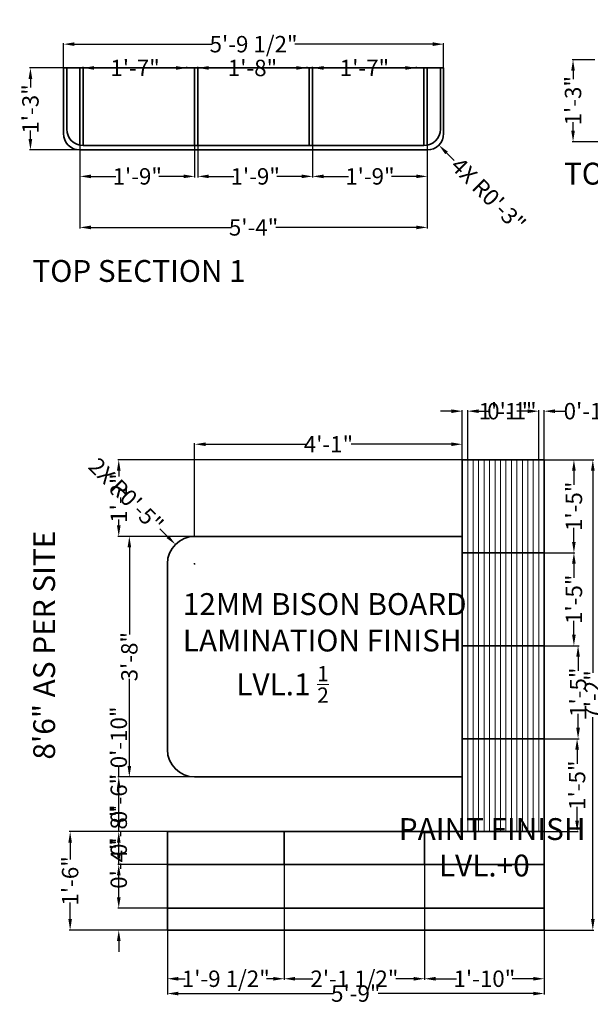
# Model space of a CAD drawing. Units: inches. Extents: x 5 to 197, y 46 to 234.
# Tile 1 of 2: x 5 to 109, y 53 to 233. Entities that reach past the tile are written whole.
import ezdxf

# ---------------------------------------------------------------- set-up
doc = ezdxf.new("R2010")
doc.units = ezdxf.units.IN
doc.header["$MEASUREMENT"] = 0
for name, color, linetype, lineweight in [('A-ANNO-DIMS', 2, 'Continuous', 18), ('A-ANNO-TEXT', 3, 'Continuous', 18), ('A-ELEV', 7, 'Continuous', 35), ('A-ELEV-PATT', 8, 'Continuous', 13), ('A-SECT', 7, 'Continuous', 35)]:
    doc.layers.add(name, color=color, linetype=linetype, lineweight=lineweight)
doc.styles.get("Standard").update_dxf_attribs({"font": 'arial.ttf'})
doc.dimstyles.get("Standard").update_dxf_attribs({"dimtxt": 3, "dimasz": 2, "dimexe": 0.18, "dimexo": 0.0625, "dimgap": 0.09, "dimtad": 0, "dimdec": 0, "dimzin": 0, "dimdsep": 46, "dimlunit": 4, "dimtxsty": 'Standard', "dimcen": 0.09, "dimadec": 0, "dimazin": 0, "dimtfac": 1, "dimtdec": 0, "dimtofl": 0, "dimtmove": 0, "dimatfit": 3, "dimfxl": 1, "dimtolj": 1, "dimtzin": 0, "dimarcsym": 1})

# ---------------------------------------------------------------- blocks, each defined once
blk = doc.blocks.new('*D1')
at = {"layer": 'A-ANNO-DIMS', "color": 0, "lineweight": -2, "transparency": 16777216}
for p, q in [((15.56, 209.27), (15.56, 194.99)), ((79.16, 209.27), (79.16, 194.99)), ((17.56, 195.17), (43.29, 195.17)), ((77.16, 195.17), (51.44, 195.17))]:
    blk.add_line(p, q, dxfattribs=at)
at = {"layer": 'A-ANNO-DIMS', "color": 0, "transparency": 16777216}
for points in [[(17.56, 195.5), (17.56, 194.83), (15.56, 195.17)], [(77.16, 195.5), (77.16, 194.83), (79.16, 195.17)]]:
    blk.add_solid(points, dxfattribs=at)
at = {"layer": 'Defpoints', "color": 0, "transparency": 16777216}
for p in [(15.56, 209.33), (79.16, 209.33), (79.16, 195.17)]:
    blk.add_point(p, dxfattribs=at)
at = {"layer": 'A-ANNO-DIMS', "color": 0, "transparency": 16777216, "insert": (47.36, 195.17), "char_height": 3, "attachment_point": 5}
blk.add_mtext('\\A1;5\'-4"', dxfattribs=at)
blk = doc.blocks.new('*D2')
at = {"layer": 'A-ANNO-DIMS', "color": 0, "lineweight": -2, "transparency": 16777216}
for p, q in [((15.56, 210.07), (15.56, 204.32)), ((36.56, 210.07), (36.56, 204.32)), ((17.56, 204.5), (22.13, 204.5)), ((34.56, 204.5), (30, 204.5))]:
    blk.add_line(p, q, dxfattribs=at)
at = {"layer": 'A-ANNO-DIMS', "color": 0, "transparency": 16777216}
for points in [[(17.56, 204.83), (17.56, 204.17), (15.56, 204.5)], [(34.56, 204.83), (34.56, 204.17), (36.56, 204.5)]]:
    blk.add_solid(points, dxfattribs=at)
at = {"layer": 'Defpoints', "color": 0, "transparency": 16777216}
for p in [(15.56, 210.13), (36.56, 210.13), (36.56, 204.5)]:
    blk.add_point(p, dxfattribs=at)
at = {"layer": 'A-ANNO-DIMS', "color": 0, "transparency": 16777216, "insert": (26.06, 204.5), "char_height": 3, "attachment_point": 5}
blk.add_mtext('\\A1;1\'-9"', dxfattribs=at)
blk = doc.blocks.new('*D3')
at = {"layer": 'A-ANNO-DIMS', "color": 0, "lineweight": -2, "transparency": 16777216}
for p, q in [((37.16, 210.07), (37.16, 204.32)), ((58.16, 210.07), (58.16, 204.32)), ((39.16, 204.5), (43.73, 204.5)), ((56.16, 204.5), (51.6, 204.5))]:
    blk.add_line(p, q, dxfattribs=at)
at = {"layer": 'A-ANNO-DIMS', "color": 0, "transparency": 16777216}
for points in [[(39.16, 204.83), (39.16, 204.17), (37.16, 204.5)], [(56.16, 204.83), (56.16, 204.17), (58.16, 204.5)]]:
    blk.add_solid(points, dxfattribs=at)
at = {"layer": 'Defpoints', "color": 0, "transparency": 16777216}
for p in [(37.16, 210.13), (58.16, 210.13), (58.16, 204.5)]:
    blk.add_point(p, dxfattribs=at)
at = {"layer": 'A-ANNO-DIMS', "color": 0, "transparency": 16777216, "insert": (47.66, 204.5), "char_height": 3, "attachment_point": 5}
blk.add_mtext('\\A1;1\'-9"', dxfattribs=at)
blk = doc.blocks.new('*D4')
at = {"layer": 'A-ANNO-DIMS', "color": 0, "lineweight": -2, "transparency": 16777216}
for p, q in [((58.16, 210.07), (58.16, 204.32)), ((79.16, 210.13), (79.16, 204.32)), ((60.16, 204.5), (64.73, 204.5)), ((77.16, 204.5), (72.6, 204.5))]:
    blk.add_line(p, q, dxfattribs=at)
at = {"layer": 'A-ANNO-DIMS', "color": 0, "transparency": 16777216}
for points in [[(60.16, 204.83), (60.16, 204.17), (58.16, 204.5)], [(77.16, 204.83), (77.16, 204.17), (79.16, 204.5)]]:
    blk.add_solid(points, dxfattribs=at)
at = {"layer": 'Defpoints', "color": 0, "transparency": 16777216}
for p in [(58.16, 210.13), (79.16, 210.19), (79.16, 204.5)]:
    blk.add_point(p, dxfattribs=at)
at = {"layer": 'A-ANNO-DIMS', "color": 0, "transparency": 16777216, "insert": (68.66, 204.5), "char_height": 3, "attachment_point": 5}
blk.add_mtext('\\A1;1\'-9"', dxfattribs=at)
blk = doc.blocks.new('*D5')
at = {"layer": 'A-ANNO-DIMS', "color": 0, "lineweight": -2, "transparency": 16777216}
for p, q in [((16.16, 224.4), (16.16, 224.51)), ((18.16, 224.33), (21.73, 224.33)), ((33.16, 224.33), (29.6, 224.33)), ((35.16, 224.4), (35.16, 224.51))]:
    blk.add_line(p, q, dxfattribs=at)
at = {"layer": 'A-ANNO-DIMS', "color": 0, "transparency": 16777216}
for points in [[(18.16, 224.67), (18.16, 224), (16.16, 224.33)], [(33.16, 224.67), (33.16, 224), (35.16, 224.33)]]:
    blk.add_solid(points, dxfattribs=at)
at = {"layer": 'Defpoints', "color": 0, "transparency": 16777216}
for p in [(16.16, 224.33), (35.16, 224.33), (35.16, 224.33)]:
    blk.add_point(p, dxfattribs=at)
at = {"layer": 'A-ANNO-DIMS', "color": 0, "transparency": 16777216, "insert": (25.66, 224.33), "char_height": 3, "attachment_point": 5}
blk.add_mtext('\\A1;1\'-7"', dxfattribs=at)
blk = doc.blocks.new('*D6')
at = {"layer": 'A-ANNO-DIMS', "color": 0, "lineweight": -2, "transparency": 16777216}
for p, q in [((37.16, 224.4), (37.16, 224.51)), ((39.16, 224.33), (43.23, 224.33)), ((55.16, 224.33), (51.1, 224.33)), ((57.16, 224.4), (57.16, 224.51))]:
    blk.add_line(p, q, dxfattribs=at)
at = {"layer": 'A-ANNO-DIMS', "color": 0, "transparency": 16777216}
for points in [[(39.16, 224.67), (39.16, 224), (37.16, 224.33)], [(55.16, 224.67), (55.16, 224), (57.16, 224.33)]]:
    blk.add_solid(points, dxfattribs=at)
at = {"layer": 'Defpoints', "color": 0, "transparency": 16777216}
for p in [(37.16, 224.33), (57.16, 224.33), (57.16, 224.33)]:
    blk.add_point(p, dxfattribs=at)
at = {"layer": 'A-ANNO-DIMS', "color": 0, "transparency": 16777216, "insert": (47.16, 224.33), "char_height": 3, "attachment_point": 5}
blk.add_mtext('\\A1;1\'-8"', dxfattribs=at)
blk = doc.blocks.new('*D7')
at = {"layer": 'A-ANNO-DIMS', "color": 0, "lineweight": -2, "transparency": 16777216}
for p, q in [((58.16, 224.4), (58.16, 224.51)), ((60.16, 224.33), (63.73, 224.33)), ((75.16, 224.33), (71.6, 224.33)), ((77.16, 224.4), (77.16, 224.51))]:
    blk.add_line(p, q, dxfattribs=at)
at = {"layer": 'A-ANNO-DIMS', "color": 0, "transparency": 16777216}
for points in [[(60.16, 224.67), (60.16, 224), (58.16, 224.33)], [(75.16, 224.67), (75.16, 224), (77.16, 224.33)]]:
    blk.add_solid(points, dxfattribs=at)
at = {"layer": 'Defpoints', "color": 0, "transparency": 16777216}
for p in [(58.16, 224.33), (77.16, 224.33), (77.16, 224.33)]:
    blk.add_point(p, dxfattribs=at)
at = {"layer": 'A-ANNO-DIMS', "color": 0, "transparency": 16777216, "insert": (67.66, 224.33), "char_height": 3, "attachment_point": 5}
blk.add_mtext('\\A1;1\'-7"', dxfattribs=at)
blk = doc.blocks.new('*D8')
at = {"layer": 'A-ANNO-DIMS', "color": 0, "lineweight": -2, "transparency": 16777216}
for p, q in [((16.1, 224.33), (6.32, 224.33)), ((6.5, 222.33), (6.5, 220.77)), ((6.5, 211.33), (6.5, 212.9)), ((15.5, 209.33), (6.32, 209.33))]:
    blk.add_line(p, q, dxfattribs=at)
at = {"layer": 'A-ANNO-DIMS', "color": 0, "transparency": 16777216}
for points in [[(6.16, 222.33), (6.83, 222.33), (6.5, 224.33)], [(6.16, 211.33), (6.83, 211.33), (6.5, 209.33)]]:
    blk.add_solid(points, dxfattribs=at)
at = {"layer": 'Defpoints', "color": 0, "transparency": 16777216}
for p in [(16.16, 224.33), (6.5, 209.33), (15.56, 209.33)]:
    blk.add_point(p, dxfattribs=at)
at = {"layer": 'A-ANNO-DIMS', "color": 0, "transparency": 16777216, "insert": (6.5, 216.83), "char_height": 3, "attachment_point": 5, "rotation": 90}
blk.add_mtext('\\A1;1\'-3"', dxfattribs=at)
blk = doc.blocks.new('*D9')
at = {"layer": 'A-ANNO-DIMS', "color": 0, "lineweight": -2, "transparency": 16777216}
for p, q in [((100.64, 135.66), (106.19, 135.66)), ((106.01, 133.66), (106.01, 131.09)), ((106.01, 120.66), (106.01, 123.22)), ((100.64, 118.66), (106.19, 118.66))]:
    blk.add_line(p, q, dxfattribs=at)
at = {"layer": 'A-ANNO-DIMS', "color": 0, "transparency": 16777216}
for points in [[(105.67, 133.66), (106.34, 133.66), (106.01, 135.66)], [(105.67, 120.66), (106.34, 120.66), (106.01, 118.66)]]:
    blk.add_solid(points, dxfattribs=at)
at = {"layer": 'Defpoints', "color": 0, "transparency": 16777216}
for p in [(100.57, 135.66), (106.01, 135.66), (100.57, 118.66)]:
    blk.add_point(p, dxfattribs=at)
at = {"layer": 'A-ANNO-DIMS', "color": 0, "transparency": 16777216, "insert": (106.01, 127.16), "char_height": 3, "attachment_point": 5, "rotation": 90}
blk.add_mtext('\\A1;1\'-5"', dxfattribs=at)
blk = doc.blocks.new('*D10')
at = {"layer": 'A-ANNO-DIMS', "color": 0, "lineweight": -2, "transparency": 16777216}
for p, q in [((100.64, 118.66), (106.95, 118.66)), ((106.77, 116.66), (106.77, 114.09)), ((106.77, 103.66), (106.77, 106.22)), ((100.64, 101.66), (106.95, 101.66))]:
    blk.add_line(p, q, dxfattribs=at)
at = {"layer": 'A-ANNO-DIMS', "color": 0, "transparency": 16777216}
for points in [[(106.44, 116.66), (107.11, 116.66), (106.77, 118.66)], [(106.44, 103.66), (107.11, 103.66), (106.77, 101.66)]]:
    blk.add_solid(points, dxfattribs=at)
at = {"layer": 'Defpoints', "color": 0, "transparency": 16777216}
for p in [(100.57, 118.66), (106.77, 118.66), (100.57, 101.66)]:
    blk.add_point(p, dxfattribs=at)
at = {"layer": 'A-ANNO-DIMS', "color": 0, "transparency": 16777216, "insert": (106.77, 110.16), "char_height": 3, "attachment_point": 5, "rotation": 90}
blk.add_mtext('\\A1;1\'-5"', dxfattribs=at)
blk = doc.blocks.new('*D11')
at = {"layer": 'A-ANNO-DIMS', "color": 0, "lineweight": -2, "transparency": 16777216}
for p, q in [((100.64, 101.66), (106.77, 101.66)), ((106.59, 99.66), (106.59, 97.09)), ((106.59, 86.66), (106.59, 89.22)), ((100.64, 84.66), (106.77, 84.66))]:
    blk.add_line(p, q, dxfattribs=at)
at = {"layer": 'A-ANNO-DIMS', "color": 0, "transparency": 16777216}
for points in [[(106.26, 99.66), (106.93, 99.66), (106.59, 101.66)], [(106.26, 86.66), (106.93, 86.66), (106.59, 84.66)]]:
    blk.add_solid(points, dxfattribs=at)
at = {"layer": 'Defpoints', "color": 0, "transparency": 16777216}
for p in [(100.57, 101.66), (106.59, 101.66), (100.57, 84.66)]:
    blk.add_point(p, dxfattribs=at)
at = {"layer": 'A-ANNO-DIMS', "color": 0, "transparency": 16777216, "insert": (106.59, 93.16), "char_height": 3, "attachment_point": 5, "rotation": 90}
blk.add_mtext('\\A1;1\'-5"', dxfattribs=at)
blk = doc.blocks.new('*D12')
at = {"layer": 'A-ANNO-DIMS', "color": 0, "lineweight": -2, "transparency": 16777216}
for p, q in [((31.57, 66.59), (31.57, 54.87)), ((100.57, 66.59), (100.57, 54.87)), ((33.57, 55.05), (62, 55.05)), ((98.57, 55.05), (70.15, 55.05))]:
    blk.add_line(p, q, dxfattribs=at)
at = {"layer": 'A-ANNO-DIMS', "color": 0, "transparency": 16777216}
for points in [[(33.57, 55.38), (33.57, 54.72), (31.57, 55.05)], [(98.57, 55.38), (98.57, 54.72), (100.57, 55.05)]]:
    blk.add_solid(points, dxfattribs=at)
at = {"layer": 'Defpoints', "color": 0, "transparency": 16777216}
for p in [(31.57, 66.66), (100.57, 66.66), (31.57, 55.05)]:
    blk.add_point(p, dxfattribs=at)
at = {"layer": 'A-ANNO-DIMS', "color": 0, "transparency": 16777216, "insert": (66.07, 55.05), "char_height": 3, "attachment_point": 5}
blk.add_mtext('\\A1;5\'-9"', dxfattribs=at)
blk = doc.blocks.new('*D13')
at = {"layer": 'A-ANNO-DIMS', "color": 0, "lineweight": -2, "transparency": 16777216}
for p, q in [((31.51, 84.66), (13.59, 84.66)), ((13.77, 82.66), (13.77, 79.59)), ((13.77, 68.66), (13.77, 71.72)), ((31.51, 66.66), (13.59, 66.66))]:
    blk.add_line(p, q, dxfattribs=at)
at = {"layer": 'A-ANNO-DIMS', "color": 0, "transparency": 16777216}
for points in [[(13.44, 82.66), (14.1, 82.66), (13.77, 84.66)], [(13.44, 68.66), (14.1, 68.66), (13.77, 66.66)]]:
    blk.add_solid(points, dxfattribs=at)
at = {"layer": 'Defpoints', "color": 0, "transparency": 16777216}
for p in [(13.77, 84.66), (31.57, 84.66), (31.57, 66.66)]:
    blk.add_point(p, dxfattribs=at)
at = {"layer": 'A-ANNO-DIMS', "color": 0, "transparency": 16777216, "insert": (13.77, 75.66), "char_height": 3, "attachment_point": 5, "rotation": 90}
blk.add_mtext('\\A1;1\'-6"', dxfattribs=at)
blk = doc.blocks.new('*D14')
at = {"layer": 'A-ANNO-DIMS', "color": 0, "lineweight": -2, "transparency": 16777216}
for p, q in [((100.64, 152.66), (106.19, 152.66)), ((106.01, 150.66), (106.01, 148.09)), ((106.01, 137.66), (106.01, 140.22)), ((100.64, 135.66), (106.19, 135.66))]:
    blk.add_line(p, q, dxfattribs=at)
at = {"layer": 'A-ANNO-DIMS', "color": 0, "transparency": 16777216}
for points in [[(105.67, 150.66), (106.34, 150.66), (106.01, 152.66)], [(105.67, 137.66), (106.34, 137.66), (106.01, 135.66)]]:
    blk.add_solid(points, dxfattribs=at)
at = {"layer": 'Defpoints', "color": 0, "transparency": 16777216}
for p in [(100.57, 152.66), (106.01, 152.66), (100.57, 135.66)]:
    blk.add_point(p, dxfattribs=at)
at = {"layer": 'A-ANNO-DIMS', "color": 0, "transparency": 16777216, "insert": (106.01, 144.16), "char_height": 3, "attachment_point": 5, "rotation": 90}
blk.add_mtext('\\A1;1\'-5"', dxfattribs=at)
blk = doc.blocks.new('*D15')
at = {"layer": 'A-ANNO-DIMS', "color": 0, "lineweight": -2, "transparency": 16777216}
for p, q in [((36.51, 138.66), (24.43, 138.66)), ((24.61, 136.66), (24.61, 120.73)), ((24.61, 96.66), (24.61, 112.58)), ((36.51, 94.66), (24.43, 94.66))]:
    blk.add_line(p, q, dxfattribs=at)
at = {"layer": 'A-ANNO-DIMS', "color": 0, "transparency": 16777216}
for points in [[(24.28, 136.66), (24.94, 136.66), (24.61, 138.66)], [(24.28, 96.66), (24.94, 96.66), (24.61, 94.66)]]:
    blk.add_solid(points, dxfattribs=at)
at = {"layer": 'Defpoints', "color": 0, "transparency": 16777216}
for p in [(36.57, 138.66), (24.61, 94.66), (36.57, 94.66)]:
    blk.add_point(p, dxfattribs=at)
at = {"layer": 'A-ANNO-DIMS', "color": 0, "transparency": 16777216, "insert": (24.61, 116.66), "char_height": 3, "attachment_point": 5, "rotation": 90}
blk.add_mtext('\\A1;3\'-8"', dxfattribs=at)
blk = doc.blocks.new('*D16')
at = {"layer": 'A-ANNO-DIMS', "color": 0, "lineweight": -2, "transparency": 16777216}
for p, q in [((36.57, 138.72), (36.57, 155.69)), ((38.57, 155.51), (56.94, 155.51)), ((83.57, 155.51), (65.21, 155.51)), ((85.57, 138.72), (85.57, 155.69))]:
    blk.add_line(p, q, dxfattribs=at)
at = {"layer": 'A-ANNO-DIMS', "color": 0, "transparency": 16777216}
for points in [[(38.57, 155.84), (38.57, 155.18), (36.57, 155.51)], [(83.57, 155.84), (83.57, 155.18), (85.57, 155.51)]]:
    blk.add_solid(points, dxfattribs=at)
at = {"layer": 'Defpoints', "color": 0, "transparency": 16777216}
for p in [(85.57, 155.51), (36.57, 138.66), (85.57, 138.66)]:
    blk.add_point(p, dxfattribs=at)
at = {"layer": 'A-ANNO-DIMS', "color": 0, "transparency": 16777216, "insert": (61.07, 155.51), "char_height": 3, "attachment_point": 5}
blk.add_mtext('\\A1;4\'-1"', dxfattribs=at)
blk = doc.blocks.new('*D17')
at = {"layer": 'A-ANNO-DIMS', "color": 0, "lineweight": -2, "transparency": 16777216}
for p, q in [((22.67, 72.66), (22.67, 74.66)), ((31.51, 70.66), (22.49, 70.66)), ((31.51, 66.66), (22.49, 66.66)), ((22.67, 64.66), (22.67, 62.66))]:
    blk.add_line(p, q, dxfattribs=at)
at = {"layer": 'A-ANNO-DIMS', "color": 0, "transparency": 16777216}
for points in [[(22.34, 72.66), (23.01, 72.66), (22.67, 70.66)], [(22.34, 64.66), (23.01, 64.66), (22.67, 66.66)]]:
    blk.add_solid(points, dxfattribs=at)
at = {"layer": 'Defpoints', "color": 0, "transparency": 16777216}
for p in [(22.67, 70.66), (31.57, 70.66), (31.57, 66.66)]:
    blk.add_point(p, dxfattribs=at)
at = {"layer": 'A-ANNO-DIMS', "color": 0, "transparency": 16777216, "insert": (22.67, 78.73), "char_height": 3, "attachment_point": 5, "rotation": 90}
blk.add_mtext('\\A1;0\'-4"', dxfattribs=at)
blk = doc.blocks.new('*D18')
at = {"layer": 'A-ANNO-DIMS', "color": 0, "lineweight": -2, "transparency": 16777216}
for p, q in [((22.67, 78.66), (22.67, 80.66)), ((31.51, 78.66), (22.49, 78.66)), ((22.67, 72.66), (22.67, 76.66)), ((31.51, 70.66), (22.49, 70.66))]:
    blk.add_line(p, q, dxfattribs=at)
at = {"layer": 'A-ANNO-DIMS', "color": 0, "transparency": 16777216}
for points in [[(22.34, 76.66), (23.01, 76.66), (22.67, 78.66)], [(22.34, 72.66), (23.01, 72.66), (22.67, 70.66)]]:
    blk.add_solid(points, dxfattribs=at)
at = {"layer": 'Defpoints', "color": 0, "transparency": 16777216}
for p in [(22.67, 78.66), (31.57, 78.66), (31.57, 70.66)]:
    blk.add_point(p, dxfattribs=at)
at = {"layer": 'A-ANNO-DIMS', "color": 0, "transparency": 16777216, "insert": (22.67, 84.73), "char_height": 3, "attachment_point": 5, "rotation": 90}
blk.add_mtext('\\A1;0\'-8"', dxfattribs=at)
blk = doc.blocks.new('*D19')
at = {"layer": 'A-ANNO-DIMS', "color": 0, "lineweight": -2, "transparency": 16777216}
for p, q in [((22.67, 84.66), (22.67, 86.66)), ((31.51, 84.66), (22.49, 84.66)), ((22.67, 80.66), (22.67, 82.66)), ((31.51, 78.66), (22.49, 78.66))]:
    blk.add_line(p, q, dxfattribs=at)
at = {"layer": 'A-ANNO-DIMS', "color": 0, "transparency": 16777216}
for points in [[(22.34, 82.66), (23.01, 82.66), (22.67, 84.66)], [(22.34, 80.66), (23.01, 80.66), (22.67, 78.66)]]:
    blk.add_solid(points, dxfattribs=at)
at = {"layer": 'Defpoints', "color": 0, "transparency": 16777216}
for p in [(22.67, 84.66), (31.57, 84.66), (31.57, 78.66)]:
    blk.add_point(p, dxfattribs=at)
at = {"layer": 'A-ANNO-DIMS', "color": 0, "transparency": 16777216, "insert": (22.67, 90.73), "char_height": 3, "attachment_point": 5, "rotation": 90}
blk.add_mtext('\\A1;0\'-6"', dxfattribs=at)
blk = doc.blocks.new('*D20')
at = {"layer": 'A-ANNO-DIMS', "color": 0, "lineweight": -2, "transparency": 16777216}
for p, q in [((22.67, 94.66), (22.67, 96.66)), ((36.51, 94.66), (22.49, 94.66)), ((22.67, 86.66), (22.67, 92.66)), ((31.51, 84.66), (22.49, 84.66))]:
    blk.add_line(p, q, dxfattribs=at)
at = {"layer": 'A-ANNO-DIMS', "color": 0, "transparency": 16777216}
for points in [[(22.34, 92.66), (23.01, 92.66), (22.67, 94.66)], [(22.34, 86.66), (23.01, 86.66), (22.67, 84.66)]]:
    blk.add_solid(points, dxfattribs=at)
at = {"layer": 'Defpoints', "color": 0, "transparency": 16777216}
for p in [(22.67, 94.66), (36.57, 94.66), (31.57, 84.66)]:
    blk.add_point(p, dxfattribs=at)
at = {"layer": 'A-ANNO-DIMS', "color": 0, "transparency": 16777216, "insert": (22.67, 101.9), "char_height": 3, "attachment_point": 5, "rotation": 90}
blk.add_mtext('\\A1;0\'-10"', dxfattribs=at)
blk = doc.blocks.new('*D21')
at = {"layer": 'A-ANNO-DIMS', "color": 0, "lineweight": -2, "transparency": 16777216}
for p, q in [((85.51, 152.66), (22.49, 152.66)), ((22.67, 150.66), (22.67, 149.59)), ((22.67, 140.66), (22.67, 141.72)), ((36.51, 138.66), (22.49, 138.66))]:
    blk.add_line(p, q, dxfattribs=at)
at = {"layer": 'A-ANNO-DIMS', "color": 0, "transparency": 16777216}
for points in [[(22.34, 150.66), (23.01, 150.66), (22.67, 152.66)], [(22.34, 140.66), (23.01, 140.66), (22.67, 138.66)]]:
    blk.add_solid(points, dxfattribs=at)
at = {"layer": 'Defpoints', "color": 0, "transparency": 16777216}
for p in [(22.67, 152.66), (85.57, 152.66), (36.57, 138.66)]:
    blk.add_point(p, dxfattribs=at)
at = {"layer": 'A-ANNO-DIMS', "color": 0, "transparency": 16777216, "insert": (22.67, 145.66), "char_height": 3, "attachment_point": 5, "rotation": 90}
blk.add_mtext('\\A1;1\'-2"', dxfattribs=at)
blk = doc.blocks.new('*D22')
at = {"layer": 'A-ANNO-DIMS', "color": 0, "lineweight": -2, "transparency": 16777216}
for p, q in [((100.64, 152.66), (109.65, 152.66)), ((109.47, 150.66), (109.47, 113.72)), ((109.47, 68.66), (109.47, 105.59)), ((100.64, 66.66), (109.65, 66.66))]:
    blk.add_line(p, q, dxfattribs=at)
at = {"layer": 'A-ANNO-DIMS', "color": 0, "transparency": 16777216}
for points in [[(109.14, 150.66), (109.81, 150.66), (109.47, 152.66)], [(109.14, 68.66), (109.81, 68.66), (109.47, 66.66)]]:
    blk.add_solid(points, dxfattribs=at)
at = {"layer": 'Defpoints', "color": 0, "transparency": 16777216}
for p in [(100.57, 152.66), (109.47, 152.66), (100.57, 66.66)]:
    blk.add_point(p, dxfattribs=at)
at = {"layer": 'A-ANNO-DIMS', "color": 0, "transparency": 16777216, "insert": (109.47, 109.66), "char_height": 3, "attachment_point": 5, "rotation": 90}
blk.add_mtext('\\A1;7\'-2"', dxfattribs=at)
blk = doc.blocks.new('*D23')
at = {"layer": 'A-ANNO-DIMS', "color": 0, "lineweight": -2, "transparency": 16777216}
for p, q in [((31.57, 84.59), (31.57, 57.58)), ((52.97, 84.59), (52.97, 57.58)), ((33.57, 57.76), (34.84, 57.76)), ((50.97, 57.76), (49.7, 57.76))]:
    blk.add_line(p, q, dxfattribs=at)
at = {"layer": 'A-ANNO-DIMS', "color": 0, "transparency": 16777216}
for points in [[(33.57, 58.09), (33.57, 57.42), (31.57, 57.76)], [(50.97, 58.09), (50.97, 57.42), (52.97, 57.76)]]:
    blk.add_solid(points, dxfattribs=at)
at = {"layer": 'Defpoints', "color": 0, "transparency": 16777216}
for p in [(31.57, 84.66), (52.97, 84.66), (52.97, 57.76)]:
    blk.add_point(p, dxfattribs=at)
at = {"layer": 'A-ANNO-DIMS', "color": 0, "transparency": 16777216, "insert": (42.27, 57.76), "char_height": 3, "attachment_point": 5}
blk.add_mtext('\\A1;1\'-9 1/2"', dxfattribs=at)
blk = doc.blocks.new('*D24')
at = {"layer": 'A-ANNO-DIMS', "color": 0, "lineweight": -2, "transparency": 16777216}
for p, q in [((52.97, 84.59), (52.97, 57.58)), ((78.67, 84.59), (78.67, 57.58)), ((54.97, 57.76), (58.22, 57.76)), ((76.67, 57.76), (73.41, 57.76))]:
    blk.add_line(p, q, dxfattribs=at)
at = {"layer": 'A-ANNO-DIMS', "color": 0, "transparency": 16777216}
for points in [[(54.97, 58.09), (54.97, 57.42), (52.97, 57.76)], [(76.67, 58.09), (76.67, 57.42), (78.67, 57.76)]]:
    blk.add_solid(points, dxfattribs=at)
at = {"layer": 'Defpoints', "color": 0, "transparency": 16777216}
for p in [(52.97, 84.66), (78.67, 84.66), (78.67, 57.76)]:
    blk.add_point(p, dxfattribs=at)
at = {"layer": 'A-ANNO-DIMS', "color": 0, "transparency": 16777216, "insert": (65.82, 57.76), "char_height": 3, "attachment_point": 5}
blk.add_mtext('\\A1;2\'-1 1/2"', dxfattribs=at)
blk = doc.blocks.new('*D25')
at = {"layer": 'A-ANNO-DIMS', "color": 0, "lineweight": -2, "transparency": 16777216}
for p, q in [((78.67, 84.59), (78.67, 57.58)), ((100.57, 84.59), (100.57, 57.58)), ((80.67, 57.76), (84.52, 57.76)), ((98.57, 57.76), (94.72, 57.76))]:
    blk.add_line(p, q, dxfattribs=at)
at = {"layer": 'A-ANNO-DIMS', "color": 0, "transparency": 16777216}
for points in [[(80.67, 58.09), (80.67, 57.42), (78.67, 57.76)], [(98.57, 58.09), (98.57, 57.42), (100.57, 57.76)]]:
    blk.add_solid(points, dxfattribs=at)
at = {"layer": 'Defpoints', "color": 0, "transparency": 16777216}
for p in [(78.67, 84.66), (100.57, 84.66), (100.57, 57.76)]:
    blk.add_point(p, dxfattribs=at)
at = {"layer": 'A-ANNO-DIMS', "color": 0, "transparency": 16777216, "insert": (89.62, 57.76), "char_height": 3, "attachment_point": 5}
blk.add_mtext('\\A1;1\'-10"', dxfattribs=at)
blk = doc.blocks.new('*D26')
at = {"layer": 'A-ANNO-DIMS', "color": 0, "lineweight": -2, "transparency": 16777216}
for p, q in [((83.57, 161.56), (81.57, 161.56)), ((85.57, 152.72), (85.57, 161.74)), ((86.57, 152.72), (86.57, 161.74)), ((88.57, 161.56), (90.57, 161.56))]:
    blk.add_line(p, q, dxfattribs=at)
at = {"layer": 'A-ANNO-DIMS', "color": 0, "transparency": 16777216}
for points in [[(83.57, 161.89), (83.57, 161.22), (85.57, 161.56)], [(88.57, 161.89), (88.57, 161.22), (86.57, 161.56)]]:
    blk.add_solid(points, dxfattribs=at)
at = {"layer": 'Defpoints', "color": 0, "transparency": 16777216}
for p in [(86.57, 161.56), (85.57, 152.66), (86.57, 152.66)]:
    blk.add_point(p, dxfattribs=at)
at = {"layer": 'A-ANNO-DIMS', "color": 0, "transparency": 16777216, "insert": (94.65, 161.56), "char_height": 3, "attachment_point": 5}
blk.add_mtext('\\A1;0\'-1"', dxfattribs=at)
blk = doc.blocks.new('*D27')
at = {"layer": 'A-ANNO-DIMS', "color": 0, "lineweight": -2, "transparency": 16777216}
for p, q in [((86.57, 152.72), (86.57, 161.74)), ((88.57, 161.56), (89.14, 161.56)), ((97.57, 161.56), (97.01, 161.56)), ((99.57, 152.72), (99.57, 161.74))]:
    blk.add_line(p, q, dxfattribs=at)
at = {"layer": 'A-ANNO-DIMS', "color": 0, "transparency": 16777216}
for points in [[(88.57, 161.89), (88.57, 161.22), (86.57, 161.56)], [(97.57, 161.89), (97.57, 161.22), (99.57, 161.56)]]:
    blk.add_solid(points, dxfattribs=at)
at = {"layer": 'Defpoints', "color": 0, "transparency": 16777216}
for p in [(99.57, 161.56), (86.57, 152.66), (99.57, 152.66)]:
    blk.add_point(p, dxfattribs=at)
at = {"layer": 'A-ANNO-DIMS', "color": 0, "transparency": 16777216, "insert": (93.07, 161.56), "char_height": 3, "attachment_point": 5}
blk.add_mtext('\\A1;1\'-1"', dxfattribs=at)
blk = doc.blocks.new('*D28')
at = {"layer": 'A-ANNO-DIMS', "color": 0, "lineweight": -2, "transparency": 16777216}
for p, q in [((97.57, 161.56), (95.57, 161.56)), ((99.57, 152.72), (99.57, 161.74)), ((100.57, 152.72), (100.57, 161.74)), ((102.57, 161.56), (104.57, 161.56))]:
    blk.add_line(p, q, dxfattribs=at)
at = {"layer": 'A-ANNO-DIMS', "color": 0, "transparency": 16777216}
for points in [[(97.57, 161.89), (97.57, 161.22), (99.57, 161.56)], [(102.57, 161.89), (102.57, 161.22), (100.57, 161.56)]]:
    blk.add_solid(points, dxfattribs=at)
at = {"layer": 'Defpoints', "color": 0, "transparency": 16777216}
for p in [(100.57, 161.56), (99.57, 152.66), (100.57, 152.66)]:
    blk.add_point(p, dxfattribs=at)
at = {"layer": 'A-ANNO-DIMS', "color": 0, "transparency": 16777216, "insert": (108.65, 161.56), "char_height": 3, "attachment_point": 5}
blk.add_mtext('\\A1;0\'-1"', dxfattribs=at)
blk = doc.blocks.new('*D29')
at = {"layer": 'A-ANNO-DIMS', "color": 0, "lineweight": -2, "transparency": 16777216}
for p, q in [((12.56, 224.4), (12.56, 228.86)), ((82.16, 224.4), (82.16, 228.86)), ((14.56, 228.68), (39.79, 228.68)), ((80.16, 228.68), (54.94, 228.68))]:
    blk.add_line(p, q, dxfattribs=at)
at = {"layer": 'A-ANNO-DIMS', "color": 0, "transparency": 16777216}
for points in [[(14.56, 229.02), (14.56, 228.35), (12.56, 228.68)], [(80.16, 229.02), (80.16, 228.35), (82.16, 228.68)]]:
    blk.add_solid(points, dxfattribs=at)
at = {"layer": 'Defpoints', "color": 0, "transparency": 16777216}
for p in [(82.16, 228.68), (12.56, 224.33), (82.16, 224.33)]:
    blk.add_point(p, dxfattribs=at)
at = {"layer": 'A-ANNO-DIMS', "color": 0, "transparency": 16777216, "insert": (47.36, 228.68), "char_height": 3, "attachment_point": 5}
blk.add_mtext('\\A1;5\'-9 1/2"', dxfattribs=at)
blk = doc.blocks.new('*D33')
at = {"layer": 'A-ANNO-DIMS', "color": 0, "lineweight": -2, "transparency": 16777216}
for p, q in [((109.84, 225.84), (105.67, 225.84)), ((105.85, 223.84), (105.85, 222.27)), ((105.85, 212.84), (105.85, 214.4)), ((112.84, 210.84), (105.67, 210.84))]:
    blk.add_line(p, q, dxfattribs=at)
at = {"layer": 'A-ANNO-DIMS', "color": 0, "transparency": 16777216}
for points in [[(105.52, 223.84), (106.18, 223.84), (105.85, 225.84)], [(105.52, 212.84), (106.18, 212.84), (105.85, 210.84)]]:
    blk.add_solid(points, dxfattribs=at)
at = {"layer": 'Defpoints', "color": 0, "transparency": 16777216}
for p in [(109.9, 225.84), (105.85, 210.84), (112.9, 210.84)]:
    blk.add_point(p, dxfattribs=at)
at = {"layer": 'A-ANNO-DIMS', "color": 0, "transparency": 16777216, "insert": (105.85, 218.34), "char_height": 3, "attachment_point": 5, "rotation": 90}
blk.add_mtext('\\A1;1\'-3"', dxfattribs=at)
blk = doc.blocks.new('*D35')
at = {"layer": 'A-ANNO-DIMS', "color": 0, "lineweight": -2, "transparency": 16777216}
for p, q in [((30.21, 140.02), (31.62, 138.61)), ((36.48, 133.66), (36.66, 133.66)), ((36.57, 133.57), (36.57, 133.75))]:
    blk.add_line(p, q, dxfattribs=at)
at = {"layer": 'A-ANNO-DIMS', "color": 0, "transparency": 16777216}
blk.add_solid([(31.86, 138.84), (31.39, 138.37), (33.04, 137.19)], dxfattribs=at)
at = {"layer": 'Defpoints', "color": 0, "transparency": 16777216}
for p in [(33.04, 137.19), (36.57, 133.66)]:
    blk.add_point(p, dxfattribs=at)
at = {"layer": 'A-ANNO-DIMS', "color": 0, "transparency": 16777216, "insert": (24.01, 146.21), "char_height": 3, "attachment_point": 5, "rotation": 315.007}
blk.add_mtext('\\A1;2X R0\'-5"', dxfattribs=at)
blk = doc.blocks.new('*D36')
at = {"layer": 'A-ANNO-DIMS', "color": 0, "lineweight": -2, "transparency": 16777216}
for p, q in [((79.07, 212.33), (79.25, 212.33)), ((79.16, 212.24), (79.16, 212.42)), ((84.11, 207.38), (82.7, 208.8))]:
    blk.add_line(p, q, dxfattribs=at)
at = {"layer": 'A-ANNO-DIMS', "color": 0, "transparency": 16777216}
blk.add_solid([(82.94, 209.03), (82.46, 208.56), (81.29, 210.21)], dxfattribs=at)
at = {"layer": 'Defpoints', "color": 0, "transparency": 16777216}
for p in [(79.16, 212.33), (81.29, 210.21)]:
    blk.add_point(p, dxfattribs=at)
at = {"layer": 'A-ANNO-DIMS', "color": 0, "transparency": 16777216, "insert": (90.34, 201.16), "char_height": 3, "attachment_point": 5, "rotation": 315.0044}
blk.add_mtext('\\A1;4X R0\'-3"', dxfattribs=at)

msp = doc.modelspace()

# ---------------------------------------------------------------- linework, layer by layer
at = {"layer": 'A-ELEV'}
for p, q in [((85.57, 152.66), (85.57, 84.66)), ((100.57, 152.66), (85.57, 152.66)), ((100.57, 135.66), (100.57, 152.66)), ((36.57, 138.66), (85.57, 138.66)), ((100.57, 135.66), (85.57, 135.66)), ((100.57, 118.66), (100.57, 135.66)), ((31.57, 133.66), (31.57, 99.66)), ((100.57, 118.66), (85.57, 118.66)), ((100.57, 101.66), (100.57, 118.66)), ((100.57, 101.66), (85.57, 101.66)), ((100.57, 84.66), (100.57, 101.66)), ((36.57, 94.66), (85.57, 94.66)), ((31.57, 66.66), (31.57, 84.66)), ((31.57, 84.66), (85.57, 84.66)), ((52.97, 84.66), (52.97, 78.66)), ((78.67, 78.66), (78.67, 84.66)), ((85.57, 84.66), (100.57, 84.66)), ((100.57, 84.66), (100.57, 66.66)), ((100.57, 78.66), (31.57, 78.66)), ((100.57, 70.66), (31.57, 70.66)), ((100.57, 66.66), (31.57, 66.66))]:
    msp.add_line(p, q, dxfattribs=at)
for centre, start, end in [((36.57, 133.66), 90, 180), ((36.57, 99.66), 180, 270)]:
    msp.add_arc(centre, 5, start, end, dxfattribs=at)
at = {"layer": 'A-ELEV-PATT'}
for p, q in [((86.57, 152.66), (86.57, 84.66)), ((87.57, 152.66), (87.57, 84.66)), ((88.57, 152.66), (88.57, 84.66)), ((89.57, 152.66), (89.57, 84.66)), ((90.57, 152.66), (90.57, 84.66)), ((91.57, 152.66), (91.57, 84.66)), ((92.57, 152.66), (92.57, 84.66)), ((93.57, 152.66), (93.57, 84.66)), ((94.57, 152.66), (94.57, 84.66)), ((95.57, 152.66), (95.57, 84.66)), ((96.57, 152.66), (96.57, 84.66)), ((97.57, 152.66), (97.57, 84.66)), ((98.57, 152.66), (98.57, 84.66)), ((99.57, 152.66), (99.57, 84.66))]:
    msp.add_line(p, q, dxfattribs=at)
at = {"layer": 'A-SECT'}
for p, q in [((82.16, 224.33), (12.56, 224.33)), ((12.56, 224.33), (12.56, 212.33)), ((13.16, 224.33), (13.16, 213.13)), ((15.56, 224.33), (15.56, 210.13)), ((16.16, 224.33), (16.16, 210.13)), ((36.56, 224.33), (36.56, 210.13)), ((37.16, 224.33), (37.16, 210.13)), ((57.56, 224.33), (57.56, 210.13)), ((58.16, 224.33), (58.16, 210.13)), ((78.56, 224.33), (78.56, 210.13)), ((79.16, 224.33), (79.16, 210.13)), ((81.56, 224.33), (81.56, 213.13)), ((82.16, 224.33), (82.16, 212.33)), ((15.56, 209.33), (79.16, 209.33)), ((16.16, 210.13), (78.56, 210.13))]:
    msp.add_line(p, q, dxfattribs=at)
for centre, start, end in [((16.16, 213.13), 180, 270), ((78.56, 213.13), 270, 0), ((15.56, 212.33), 180, 270), ((79.16, 212.33), 270, 0)]:
    msp.add_arc(centre, 3, start, end, dxfattribs=at)

# ---------------------------------------------------------------- texts
at = {"layer": 'A-ANNO-TEXT', "char_height": 4, "attachment_point": 1}
for s, width, insert in [('TOP SECTION 2', 72.0117, (104.18, 207)), ('TOP SECTION 1', 52.888, (6.86, 189.2)), ('\\A1;12MM BISON BOARD\\PLAMINATION FINISH\\P        LVL.1 {\\H0.7x;\\S1/2;}', 125.0016, (34.4, 128.28)), ('PAINT FINISH \\P      LVL.+0', 80.2681, (73.95, 87.13))]:
    msp.add_mtext_dynamic_manual_height_columns(s, width=width, gutter_width=20, heights=[0], dxfattribs=dict(at, insert=insert))
at = {"layer": 'A-ANNO-TEXT', "insert": (7.01, 97.84), "char_height": 4, "attachment_point": 1, "rotation": 90}
msp.add_mtext_dynamic_manual_height_columns('8\'6" AS PER SITE', width=115.2159, gutter_width=20, heights=[0], dxfattribs=at)

# ---------------------------------------------------------------- dimensions: what is measured, and where the dimension line sits
at = {"layer": 'A-ANNO-DIMS'}
for base, p1, p2, override, picture, middle in [((82.16, 228.68), (12.56, 224.33), (82.16, 224.33), {"dimdec": 1, "dimlfac": 1, "dimrnd": 0, "dimzin": 1, "dimdsep": 46, "dimlunit": 4, "dimfrac": 2}, '*D29', (47.36, 228.68)), ((35.16, 224.33), (16.16, 224.33), (35.16, 224.33), {"dimclrd": 0, "dimclre": 0, "dimclrt": 0}, '*D5', (25.66, 224.33)), ((57.16, 224.33), (37.16, 224.33), (57.16, 224.33), {"dimclrd": 0, "dimclre": 0, "dimclrt": 0}, '*D6', (47.16, 224.33)), ((77.16, 224.33), (58.16, 224.33), (77.16, 224.33), {"dimclrd": 0, "dimclre": 0, "dimclrt": 0}, '*D7', (67.66, 224.33)), ((36.56, 204.5), (15.56, 210.13), (36.56, 210.13), {"dimclrd": 0, "dimclre": 0, "dimclrt": 0}, '*D2', (26.06, 204.5)), ((79.16, 195.17), (15.56, 209.33), (79.16, 209.33), {"dimclrd": 0, "dimclre": 0, "dimclrt": 0}, '*D1', (47.36, 195.17)), ((58.16, 204.5), (37.16, 210.13), (58.16, 210.13), {"dimclrd": 0, "dimclre": 0, "dimclrt": 0}, '*D3', (47.66, 204.5)), ((79.16, 204.5), (58.16, 210.13), (79.16, 210.19), {"dimclrd": 0, "dimclre": 0, "dimclrt": 0}, '*D4', (68.66, 204.5)), ((86.57, 161.56), (85.57, 152.66), (86.57, 152.66), {"dimdec": 1, "dimlfac": 1, "dimrnd": 0, "dimzin": 1, "dimdsep": 46, "dimlunit": 4, "dimfrac": 2}, '*D26', (94.65, 161.56)), ((99.57, 161.56), (86.57, 152.66), (99.57, 152.66), {"dimdec": 1, "dimlfac": 1, "dimrnd": 0, "dimzin": 1, "dimdsep": 46, "dimlunit": 4, "dimfrac": 2}, '*D27', (93.07, 161.56)), ((100.57, 161.56), (99.57, 152.66), (100.57, 152.66), {"dimdec": 1, "dimlfac": 1, "dimrnd": 0, "dimzin": 1, "dimdsep": 46, "dimlunit": 4, "dimfrac": 2}, '*D28', (108.65, 161.56)), ((85.57, 155.51), (36.57, 138.66), (85.57, 138.66), {"dimclrd": 0, "dimclre": 0, "dimclrt": 0}, '*D16', (61.07, 155.51)), ((52.97, 57.76), (31.57, 84.66), (52.97, 84.66), {"dimdec": 1, "dimlfac": 1, "dimrnd": 0, "dimzin": 1, "dimdsep": 46, "dimlunit": 4, "dimfrac": 2}, '*D23', (42.27, 57.76)), ((78.67, 57.76), (52.97, 84.66), (78.67, 84.66), {"dimdec": 1, "dimlfac": 1, "dimrnd": 0, "dimzin": 1, "dimdsep": 46, "dimlunit": 4, "dimfrac": 2}, '*D24', (65.82, 57.76)), ((100.57, 57.76), (78.67, 84.66), (100.57, 84.66), {"dimdec": 1, "dimlfac": 1, "dimrnd": 0, "dimzin": 1, "dimdsep": 46, "dimlunit": 4, "dimfrac": 2}, '*D25', (89.62, 57.76)), ((31.57, 55.05), (100.57, 66.66), (31.57, 66.66), {"dimclrd": 0, "dimclre": 0, "dimclrt": 0}, '*D12', (66.07, 55.05))]:
    dim = msp.add_linear_dim(base=base, p1=p1, p2=p2, dimstyle='Standard', override=override, dxfattribs=at)
    dim.commit()
    dim.dimension.update_dxf_attribs({"geometry": picture, "text_midpoint": middle})
for base, p1, p2, override, picture, middle in [((105.85, 210.84), (109.9, 225.84), (112.9, 210.84), {"dimdec": 1, "dimlfac": 1, "dimrnd": 0, "dimzin": 1, "dimdsep": 46, "dimlunit": 4, "dimfrac": 2}, '*D33', (105.85, 218.34)), ((6.5, 209.33), (16.16, 224.33), (15.56, 209.33), {"dimclrd": 0, "dimclre": 0, "dimclrt": 0}, '*D8', (6.5, 216.83)), ((22.67, 152.66), (36.57, 138.66), (85.57, 152.66), {"dimdec": 1, "dimlfac": 1, "dimrnd": 0, "dimzin": 1, "dimdsep": 46, "dimlunit": 4, "dimfrac": 2}, '*D21', (22.67, 145.66)), ((106.01, 152.66), (100.57, 135.66), (100.57, 152.66), {"dimclrd": 0, "dimclre": 0, "dimclrt": 0}, '*D14', (106.01, 144.16)), ((109.47, 152.66), (100.57, 66.66), (100.57, 152.66), {"dimdec": 1, "dimlfac": 1, "dimrnd": 0, "dimzin": 1, "dimdsep": 46, "dimlunit": 4, "dimfrac": 2}, '*D22', (109.47, 109.66)), ((24.61, 94.66), (36.57, 138.66), (36.57, 94.66), {"dimclrd": 0, "dimclre": 0, "dimclrt": 0}, '*D15', (24.61, 116.66)), ((106.01, 135.66), (100.57, 118.66), (100.57, 135.66), {"dimclrd": 0, "dimclre": 0, "dimclrt": 0}, '*D9', (106.01, 127.16)), ((106.77, 118.66), (100.57, 101.66), (100.57, 118.66), {"dimclrd": 0, "dimclre": 0, "dimclrt": 0}, '*D10', (106.77, 110.16)), ((22.67, 94.66), (31.57, 84.66), (36.57, 94.66), {"dimdec": 1, "dimlfac": 1, "dimrnd": 0, "dimzin": 1, "dimdsep": 46, "dimlunit": 4, "dimfrac": 2}, '*D20', (22.67, 101.9)), ((106.59, 101.66), (100.57, 84.66), (100.57, 101.66), {"dimclrd": 0, "dimclre": 0, "dimclrt": 0}, '*D11', (106.59, 93.16)), ((22.67, 84.66), (31.57, 78.66), (31.57, 84.66), {"dimdec": 1, "dimlfac": 1, "dimrnd": 0, "dimzin": 1, "dimdsep": 46, "dimlunit": 4, "dimfrac": 2}, '*D19', (22.67, 90.73)), ((22.67, 78.66), (31.57, 70.66), (31.57, 78.66), {"dimdec": 1, "dimlfac": 1, "dimrnd": 0, "dimzin": 1, "dimdsep": 46, "dimlunit": 4, "dimfrac": 2}, '*D18', (22.67, 84.73)), ((13.77, 84.66), (31.57, 66.66), (31.57, 84.66), {"dimclrd": 0, "dimclre": 0, "dimclrt": 0}, '*D13', (13.77, 75.66)), ((22.67, 70.66), (31.57, 66.66), (31.57, 70.66), {"dimdec": 1, "dimlfac": 1, "dimrnd": 0, "dimzin": 1, "dimdsep": 46, "dimlunit": 4, "dimfrac": 2}, '*D17', (22.67, 78.73))]:
    dim = msp.add_linear_dim(base=base, p1=p1, p2=p2, angle=90, dimstyle='Standard', override=override, dxfattribs=at)
    dim.commit()
    dim.dimension.update_dxf_attribs({"geometry": picture, "text_midpoint": middle})
for center, mpoint, text, picture, middle in [((79.16, 212.33), (81.29, 210.21), '4X <>', '*D36', (90.34, 201.16)), ((36.57, 133.66), (33.04, 137.19), '2X <>', '*D35', (24.01, 146.21))]:
    dim = msp.add_radius_dim(center=center, mpoint=mpoint, text=text, dimstyle='Standard', override={"dimdec": 1, "dimlfac": 1, "dimrnd": 0, "dimzin": 1, "dimdsep": 46, "dimlunit": 4, "dimfrac": 2}, dxfattribs=at)
    dim.commit()
    dim.dimension.update_dxf_attribs({"geometry": picture, "text_midpoint": middle})

doc.saveas('drawing.dxf')
